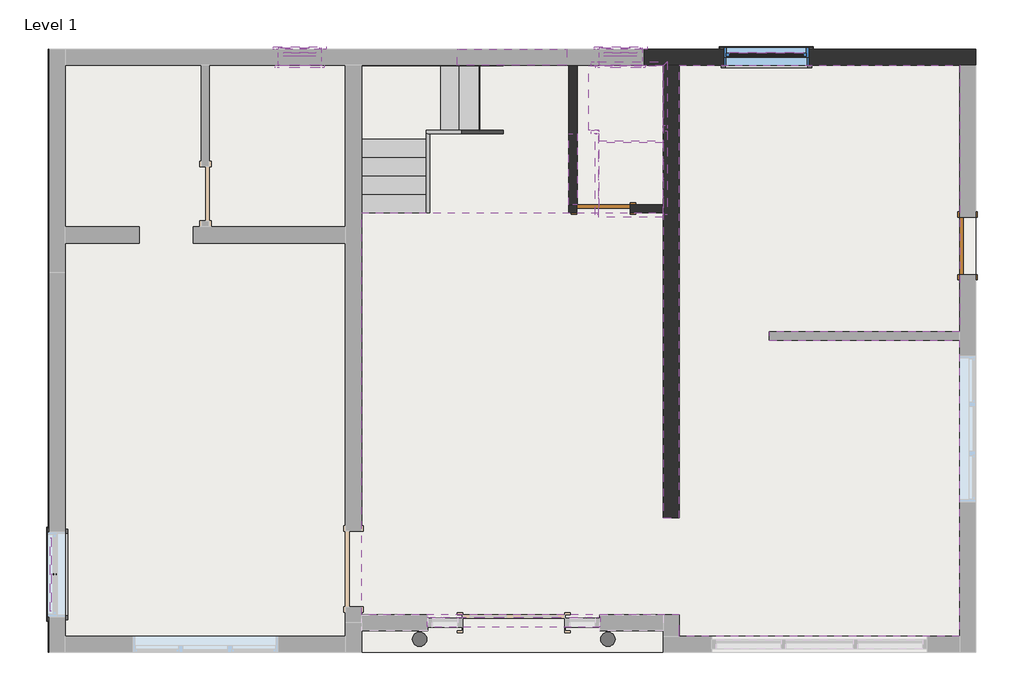
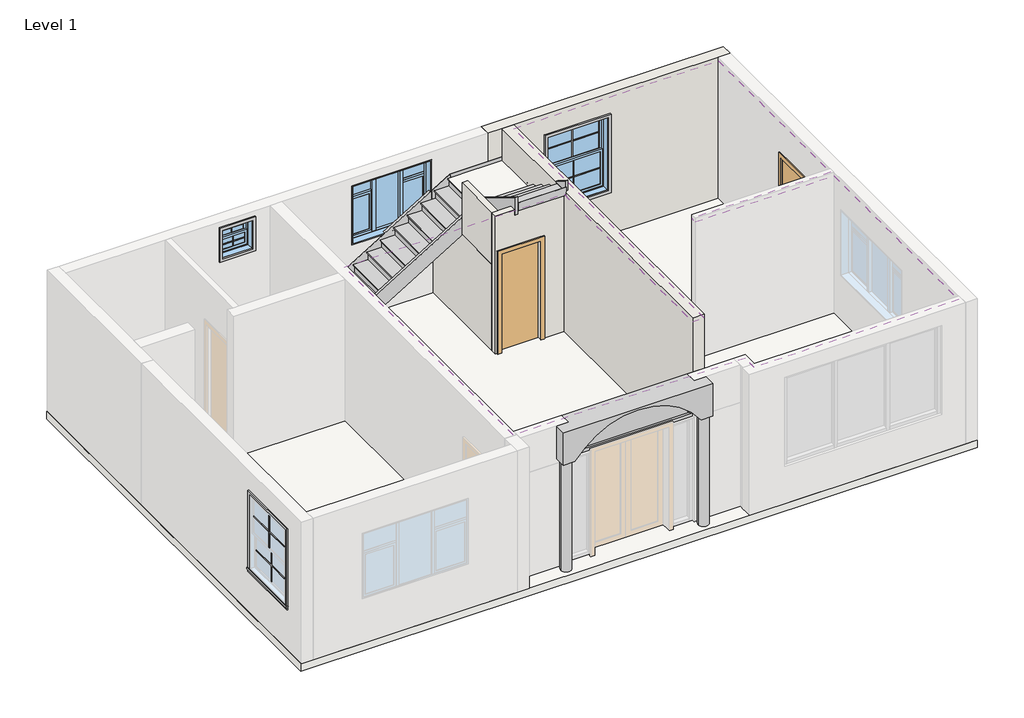
# One storey, part 2 of 2: 18 proxies, 11 members, 5 walls, 4 windows, 3 slabs, 3 stair flights, 2 doors, 1 covering.
"""IFC4 building model written with IfcOpenShell, lengths in millimetres."""

from ifc_helpers import new_model, si_unit, frame, origin, place, context, project, spatial, polyline, outline, extrude, faceted_brep, transform, mapped, element, save
from components import generic_models_1_generic_models_1_1dae4af3, generic_models_2_generic_models_2_701112c8, muntin_pattern_2x2_muntin_pattern_2x2_872d1288, muntin_pattern_2x2_muntin_pattern_2x2_cfeb24ad, trim_window_exterior_flat_with_sill_c3105ee7, trim_window_exterior_flat_with_sill_858dc10d, trim_window_interior_flat_picture_frame_d5efd988, trim_window_interior_flat_picture_frame_3927330c, door_f2b275c1, door_7b345704, non_monolithic_landing_e8e8d04f, non_monolithic_landing_bb3beaf2, stair_flight_8f72ff29, stair_flight_55fbbb17, stair_flight_157d76c2, window_1a7cbd99, window_double_hung_2_x2_15b2d83c, window_double_hung_3_11_b20011b0

model = new_model("IFC4")

# Units and contexts
model_context = context("Model", 3, world=origin())
ifc_project = project(units=[si_unit("LENGTHUNIT", "METRE", prefix="MILLI")], contexts=[model_context])

# Site, building, storey
site = spatial("IfcSite", under=ifc_project)
building = spatial("IfcBuilding", under=site)
storey = spatial("IfcBuildingStorey", under=building, Name="Level 1", Elevation=0.0)

# Proxies
placement = place(None, origin())
generic_models_1_generic_models_1_shape = generic_models_1_generic_models_1_1dae4af3(model_context)
element("IfcBuildingElementProxy", 1, Name="Generic Models 1 : Generic Models 1", ObjectType="Generic Models 1 : Generic Models 1", at=placement, inside=storey, context=model_context, shape_type="MappedRepresentation", body=[
    mapped(generic_models_1_generic_models_1_shape, transform((0.0, 0.0, 0.0), x_axis=(1.0, 0.0, 0.0), y_axis=(0.0, 1.0, 0.0), z_axis=(0.0, 0.0, 1.0))),
])
generic_models_2_generic_models_2_shape = generic_models_2_generic_models_2_701112c8(model_context)
element("IfcBuildingElementProxy", 2, Name="Generic Models 2 : Generic Models 2", ObjectType="Generic Models 2 : Generic Models 2", at=placement, inside=storey, context=model_context, shape_type="MappedRepresentation", body=[
    mapped(generic_models_2_generic_models_2_shape, transform((0.0, 0.0, 0.0), x_axis=(1.0, 0.0, 0.0), y_axis=(0.0, 1.0, 0.0), z_axis=(0.0, 0.0, 1.0))),
])
muntin_pattern_2x2_muntin_pattern_2x2_shape = muntin_pattern_2x2_muntin_pattern_2x2_872d1288(model_context)
element("IfcBuildingElementProxy", 3, Name="Muntin Pattern_2x2 : Muntin Pattern_2x2", ObjectType="Muntin Pattern_2x2 : Muntin Pattern_2x2", at=placement, inside=storey, context=model_context, shape_type="MappedRepresentation", body=[
    mapped(muntin_pattern_2x2_muntin_pattern_2x2_shape, transform((-19390.8072207, 4603.0962903, 1698.625), x_axis=(0.0, 1.0, 0.0), y_axis=(-1.0, 0.0, 0.0), z_axis=(0.0, 0.0, 1.0))),
])
element("IfcBuildingElementProxy", 4, Name="Muntin Pattern_2x2 : Muntin Pattern_2x2", ObjectType="Muntin Pattern_2x2 : Muntin Pattern_2x2", at=placement, inside=storey, context=model_context, shape_type="MappedRepresentation", body=[
    mapped(muntin_pattern_2x2_muntin_pattern_2x2_shape, transform((-19346.3572207, 4603.0962903, 990.6), x_axis=(0.0, 1.0, 0.0), y_axis=(-1.0, 0.0, 0.0), z_axis=(0.0, 0.0, 1.0))),
])
element("IfcBuildingElementProxy", 5, Name="Muntin Pattern_2x2 : Muntin Pattern_2x2", ObjectType="Muntin Pattern_2x2 : Muntin Pattern_2x2", at=placement, inside=storey, context=model_context, shape_type="MappedRepresentation", body=[
    mapped(muntin_pattern_2x2_muntin_pattern_2x2_shape, transform((-9277.2026022, 11998.6707578, 1698.625), x_axis=(1.0, 0.0, 0.0), y_axis=(0.0, 1.0, 0.0), z_axis=(0.0, 0.0, 1.0))),
])
element("IfcBuildingElementProxy", 6, Name="Muntin Pattern_2x2 : Muntin Pattern_2x2", ObjectType="Muntin Pattern_2x2 : Muntin Pattern_2x2", at=placement, inside=storey, context=model_context, shape_type="MappedRepresentation", body=[
    mapped(muntin_pattern_2x2_muntin_pattern_2x2_shape, transform((-9277.2026022, 11954.2207578, 990.6), x_axis=(1.0, 0.0, 0.0), y_axis=(0.0, 1.0, 0.0), z_axis=(0.0, 0.0, 1.0))),
])
muntin_pattern_2x2_muntin_pattern_2x2_2_shape = muntin_pattern_2x2_muntin_pattern_2x2_cfeb24ad(model_context)
element("IfcBuildingElementProxy", 7, Name="Muntin Pattern_2x2 : Muntin Pattern_2x2", ObjectType="Muntin Pattern_2x2 : Muntin Pattern_2x2", at=placement, inside=storey, context=model_context, shape_type="MappedRepresentation", body=[
    mapped(muntin_pattern_2x2_muntin_pattern_2x2_2_shape, transform((-15881.0556236, 11998.6707578, 2460.625), x_axis=(1.0, 0.0, 0.0), y_axis=(0.0, 1.0, 0.0), z_axis=(0.0, 0.0, 1.0))),
])
element("IfcBuildingElementProxy", 8, Name="Muntin Pattern_2x2 : Muntin Pattern_2x2", ObjectType="Muntin Pattern_2x2 : Muntin Pattern_2x2", at=placement, inside=storey, context=model_context, shape_type="MappedRepresentation", body=[
    mapped(muntin_pattern_2x2_muntin_pattern_2x2_2_shape, transform((-15881.0556236, 11954.2207578, 2209.8), x_axis=(1.0, 0.0, 0.0), y_axis=(0.0, 1.0, 0.0), z_axis=(0.0, 0.0, 1.0))),
])
element("IfcBuildingElementProxy", 9, Name="Muntin Pattern_2x2 : Muntin Pattern_2x2", ObjectType="Muntin Pattern_2x2 : Muntin Pattern_2x2", at=placement, inside=storey, context=model_context, shape_type="MappedRepresentation", body=[
    mapped(muntin_pattern_2x2_muntin_pattern_2x2_2_shape, transform((-11339.7531945, 11998.6707578, 1851.025), x_axis=(1.0, 0.0, 0.0), y_axis=(0.0, 1.0, 0.0), z_axis=(0.0, 0.0, 1.0))),
])
element("IfcBuildingElementProxy", 10, Name="Muntin Pattern_2x2 : Muntin Pattern_2x2", ObjectType="Muntin Pattern_2x2 : Muntin Pattern_2x2", at=placement, inside=storey, context=model_context, shape_type="MappedRepresentation", body=[
    mapped(muntin_pattern_2x2_muntin_pattern_2x2_2_shape, transform((-11339.7531945, 11954.2207578, 1600.2), x_axis=(1.0, 0.0, 0.0), y_axis=(0.0, 1.0, 0.0), z_axis=(0.0, 0.0, 1.0))),
])
trim_window_exterior_flat_with_sill_shape = trim_window_exterior_flat_with_sill_c3105ee7(model_context)
element("IfcBuildingElementProxy", 11, Name="Trim-Window-Exterior-Flat : with Sill", ObjectType="Trim-Window-Exterior-Flat : with Sill", at=placement, inside=storey, context=model_context, shape_type="MappedRepresentation", body=[
    mapped(trim_window_exterior_flat_with_sill_shape, transform((-19425.7322207, 4603.0962903, 2438.4), x_axis=(0.0, -1.0, 0.0), y_axis=(0.0, 0.0, 1.0), z_axis=(-1.0, 0.0, 0.0))),
])
element("IfcBuildingElementProxy", 12, Name="Trim-Window-Exterior-Flat : with Sill", ObjectType="Trim-Window-Exterior-Flat : with Sill", at=placement, inside=storey, context=model_context, shape_type="MappedRepresentation", body=[
    mapped(trim_window_exterior_flat_with_sill_shape, transform((-9277.2026022, 12033.5957578, 2438.4), x_axis=(-1.0, 0.0, 0.0), y_axis=(0.0, 0.0, 1.0), z_axis=(0.0, 1.0, 0.0))),
])
trim_window_exterior_flat_with_sill_2_shape = trim_window_exterior_flat_with_sill_858dc10d(model_context)
element("IfcBuildingElementProxy", 13, Name="Trim-Window-Exterior-Flat : with Sill", ObjectType="Trim-Window-Exterior-Flat : with Sill", at=placement, inside=storey, context=model_context, shape_type="MappedRepresentation", body=[
    mapped(trim_window_exterior_flat_with_sill_2_shape, transform((-15881.0556236, 12033.5957578, 2743.2), x_axis=(-1.0, 0.0, 0.0), y_axis=(0.0, 0.0, 1.0), z_axis=(0.0, 1.0, 0.0))),
])
element("IfcBuildingElementProxy", 14, Name="Trim-Window-Exterior-Flat : with Sill", ObjectType="Trim-Window-Exterior-Flat : with Sill", at=placement, inside=storey, context=model_context, shape_type="MappedRepresentation", body=[
    mapped(trim_window_exterior_flat_with_sill_2_shape, transform((-11339.7531945, 12033.5957578, 2133.6), x_axis=(-1.0, 0.0, 0.0), y_axis=(0.0, 0.0, 1.0), z_axis=(0.0, 1.0, 0.0))),
])
trim_window_interior_flat_picture_frame_shape = trim_window_interior_flat_picture_frame_d5efd988(model_context)
element("IfcBuildingElementProxy", 15, Name="Trim-Window-Interior-Flat : Picture Frame", ObjectType="Trim-Window-Interior-Flat : Picture Frame", at=placement, inside=storey, context=model_context, shape_type="MappedRepresentation", body=[
    mapped(trim_window_interior_flat_picture_frame_shape, transform((-19197.1322207, 4603.0962903, 2438.4), x_axis=(0.0, 1.0, 0.0), y_axis=(0.0, 0.0, 1.0), z_axis=(1.0, 0.0, 0.0))),
])
element("IfcBuildingElementProxy", 16, Name="Trim-Window-Interior-Flat : Picture Frame", ObjectType="Trim-Window-Interior-Flat : Picture Frame", at=placement, inside=storey, context=model_context, shape_type="MappedRepresentation", body=[
    mapped(trim_window_interior_flat_picture_frame_shape, transform((-9277.2026022, 11804.9957578, 2438.4), x_axis=(1.0, 0.0, 0.0), y_axis=(0.0, 0.0, 1.0), z_axis=(0.0, -1.0, 0.0))),
])
trim_window_interior_flat_picture_frame_2_shape = trim_window_interior_flat_picture_frame_3927330c(model_context)
element("IfcBuildingElementProxy", 17, Name="Trim-Window-Interior-Flat : Picture Frame", ObjectType="Trim-Window-Interior-Flat : Picture Frame", at=placement, inside=storey, context=model_context, shape_type="MappedRepresentation", body=[
    mapped(trim_window_interior_flat_picture_frame_2_shape, transform((-15881.0556236, 11804.9957578, 2743.2), x_axis=(1.0, 0.0, 0.0), y_axis=(0.0, 0.0, 1.0), z_axis=(0.0, -1.0, 0.0))),
])
element("IfcBuildingElementProxy", 18, Name="Trim-Window-Interior-Flat : Picture Frame", ObjectType="Trim-Window-Interior-Flat : Picture Frame", at=placement, inside=storey, context=model_context, shape_type="MappedRepresentation", body=[
    mapped(trim_window_interior_flat_picture_frame_2_shape, transform((-11339.7531945, 11804.9957578, 2133.6), x_axis=(1.0, 0.0, 0.0), y_axis=(0.0, 0.0, 1.0), z_axis=(0.0, -1.0, 0.0))),
])

# Covering
element("IfcCovering", 19, ObjectType="2' x 4' ACT System", at=placement, inside=storey, context=model_context, shape_type="SweptSolid", body=[
    extrude(outline(polyline([(-19197.1322207, 9290.2207935), (-18149.1852461, 9290.2207935), (-18149.1852461, 9518.8207935), (-19197.1322207, 9518.8207935), (-19197.1322207, 11804.9957578), (-17272.3740665, 11804.9957578), (-17272.3740665, 9518.8207935), (-17388.0183685, 9518.8207935), (-17388.0183685, 9290.2207935), (-15233.3556236, 9290.2207935), (-15233.3556236, 3726.7962903), (-19197.1322207, 3726.7962903), (-19197.1322207, 9290.2207935)])), frame((0.0, 0.0, 2819.4), z_axis=(0.0, 0.0, 1.0), x_axis=(1.0, 0.0, 0.0)), (0.0, 0.0, 1.0), 57.15),
    extrude(outline(polyline([(-6543.9817031, 11804.9957578), (-6543.9817031, 8032.8333114), (-9237.1629596, 8032.8333114), (-9237.1629596, 7918.5333114), (-6545.326005, 7918.5333114), (-6545.326005, 3726.7962903), (-10507.7583002, 3726.7962903), (-10507.7583002, 4031.4170165), (-15004.7556236, 4031.4170165), (-15004.7556236, 9720.1872586), (-10737.7026022, 9720.1872586), (-10737.7026022, 5401.1206207), (-10509.1026022, 5401.1206207), (-10509.1026022, 11804.9957578), (-6543.9817031, 11804.9957578)])), frame((0.0, 0.0, 2819.4), z_axis=(0.0, 0.0, 1.0), x_axis=(1.0, 0.0, 0.0)), (0.0, 0.0, 1.0), 57.15),
])

# Doors
door_shape = door_f2b275c1(model_context)
element("IfcDoor", 20, ObjectType="Single-Flush : 30\" x 80\"", at=placement, inside=storey, context=model_context, shape_type="MappedRepresentation", body=[
    mapped(door_shape, transform((-11582.1099332, 9778.180515, 0.0), x_axis=(-1.0, 0.0, 0.0), y_axis=(0.0, -1.0, 0.0), z_axis=(0.0, 0.0, 1.0))),
])
door_2_shape = door_7b345704(model_context)
element("IfcDoor", 21, ObjectType="Single-Flush : 32\" x 84\"", at=placement, inside=storey, context=model_context, shape_type="MappedRepresentation", body=[
    mapped(door_2_shape, transform((-6429.6817031, 9252.2957578, 0.0), x_axis=(0.0, -1.0, 0.0), y_axis=(1.0, 0.0, 0.0), z_axis=(0.0, 0.0, 1.0))),
])

# Members
element("IfcMember", 22, ObjectType="Stringer - 2\" Width", at=placement, inside=storey, context=model_context, shape_type="SweptSolid", body=[
    extrude(outline(polyline([(9720.1872586, 0.0), (9720.1872586, 212.7786153), (10805.6326245, 878.3052632), (10891.6353161, 573.5052632), (9956.2728747, 0.0), (9720.1872586, 0.0)])), frame((-15055.3982861, 0.0, 0.0), z_axis=(1.0, 0.0, 0.0), x_axis=(0.0, 1.0, 0.0)), (0.0, 0.0, 1.0), 50.8),
])
element("IfcMember", 23, ObjectType="Stringer - 2\" Width", at=placement, inside=storey, context=model_context, shape_type="SweptSolid", body=[
    extrude(outline(polyline([(9720.1872586, 0.0), (9720.1872586, 212.7786153), (10838.2453953, 898.3013576), (10838.2453953, 540.7699306), (9956.2728747, 0.0), (9720.1872586, 0.0)])), frame((-14090.1982861, 0.0, 0.0), z_axis=(1.0, 0.0, 0.0), x_axis=(0.0, 1.0, 0.0)), (0.0, 0.0, 1.0), 50.8),
])
element("IfcMember", 24, ObjectType="Stringer - 2\" Width", at=placement, inside=storey, context=model_context, shape_type="SweptSolid", body=[
    extrude(outline(polyline([(878.3052632, -14109.3311056), (573.5052632, -14023.328414), (2017.2947368, -11668.5698202), (2322.0947368, -11754.5725119), (878.3052632, -14109.3311056)])), frame((0.0, 11803.4453953, 0.0), z_axis=(0.0, 1.0, 0.0), x_axis=(0.0, 0.0, 1.0)), (0.0, 0.0, 1.0), 50.8),
])
element("IfcMember", 25, ObjectType="Stringer - 2\" Width", at=placement, inside=storey, context=model_context, shape_type="SweptSolid", body=[
    extrude(outline(polyline([(890.0363015, -14090.1982861), (532.5048745, -14090.1982861), (2017.2947368, -11668.5698202), (2322.0947368, -11754.5725119), (890.0363015, -14090.1982861)])), frame((0.0, 10838.2453953, 0.0), z_axis=(0.0, 1.0, 0.0), x_axis=(0.0, 0.0, 1.0)), (0.0, 0.0, 1.0), 50.8),
])
element("IfcMember", 26, ObjectType="Stringer - 2\" Width", at=placement, inside=storey, context=model_context, shape_type="Brep", body=[
    faceted_brep([(-14109.3311056, 11803.4453953, 878.3052632), (-14109.3311056, 11854.2453953, 878.3052632), (-15055.3982861, 11854.2453953, 878.3052632), (-15004.5982861, 11803.4453953, 878.3052632), (-14023.328414, 11803.4453953, 573.5052632), (-15004.5982861, 11803.4453953, 573.5052632), (-14023.328414, 11854.2453953, 573.5052632), (-15055.3982861, 11854.2453953, 573.5052632)], [[[0, 1, 2, 3]], [[4, 0, 3, 5]], [[6, 4, 5, 7]], [[1, 6, 7, 2]], [[1, 0, 4, 6]], [[2, 7, 5, 3]]]),
])
element("IfcMember", 27, ObjectType="Stringer - 2\" Width", at=placement, inside=storey, context=model_context, shape_type="Brep", body=[
    faceted_brep([(-15004.5982861, 11803.4453953, 878.3052632), (-15055.3982861, 11854.2453953, 878.3052632), (-15055.3982861, 10805.6326245, 878.3052632), (-15004.5982861, 10805.6326245, 878.3052632), (-15004.5982861, 11803.4453953, 573.5052632), (-15004.5982861, 10891.6353161, 573.5052632), (-15055.3982861, 11854.2453953, 573.5052632), (-15055.3982861, 10891.6353161, 573.5052632)], [[[0, 1, 2, 3]], [[4, 0, 3, 5]], [[6, 4, 5, 7]], [[1, 6, 7, 2]], [[1, 0, 4, 6]], [[2, 7, 5, 3]]]),
])
element("IfcMember", 28, ObjectType="Stringer - 2\" Width", at=placement, inside=storey, context=model_context, shape_type="SweptSolid", body=[
    extrude(outline(polyline([(10959.0950804, 2322.0947368), (10873.0923887, 2017.2947368), (9689.7818525, 2742.8261356), (9689.7818525, 3100.3575626), (10959.0950804, 2322.0947368)])), frame((-10733.9149392, 0.0, 0.0), z_axis=(1.0, 0.0, 0.0), x_axis=(0.0, 1.0, 0.0)), (0.0, 0.0, 1.0), 50.8),
])
element("IfcMember", 29, ObjectType="Stringer - 2\" Width", at=placement, inside=storey, context=model_context, shape_type="SweptSolid", body=[
    extrude(outline(polyline([(10838.2453953, 2396.1921427), (10838.2453953, 2038.6607157), (9689.7818525, 2742.8261356), (9689.7818525, 3100.3575626), (10838.2453953, 2396.1921427)])), frame((-11699.1149392, 0.0, 0.0), z_axis=(1.0, 0.0, 0.0), x_axis=(0.0, 1.0, 0.0)), (0.0, 0.0, 1.0), 50.8),
])
element("IfcMember", 30, ObjectType="Stringer - 2\" Width", at=placement, inside=storey, context=model_context, shape_type="Brep", body=[
    faceted_brep([(-10733.9149392, 10959.0950804, 2322.0947368), (-10683.1149392, 10959.0950804, 2322.0947368), (-10683.1149392, 11854.2453953, 2322.0947368), (-10733.9149392, 11803.4453953, 2322.0947368), (-10733.9149392, 10873.0923887, 2017.2947368), (-10733.9149392, 11803.4453953, 2017.2947368), (-10683.1149392, 10873.0923887, 2017.2947368), (-10683.1149392, 11854.2453953, 2017.2947368)], [[[0, 1, 2, 3]], [[4, 0, 3, 5]], [[6, 4, 5, 7]], [[1, 6, 7, 2]], [[1, 0, 4, 6]], [[2, 7, 5, 3]]]),
])
element("IfcMember", 31, ObjectType="Stringer - 2\" Width", at=placement, inside=storey, context=model_context, shape_type="Brep", body=[
    faceted_brep([(-10733.9149392, 11803.4453953, 2322.0947368), (-10683.1149392, 11854.2453953, 2322.0947368), (-11754.5725119, 11854.2453953, 2322.0947368), (-11754.5725119, 11803.4453953, 2322.0947368), (-10733.9149392, 11803.4453953, 2017.2947368), (-11668.5698202, 11803.4453953, 2017.2947368), (-10683.1149392, 11854.2453953, 2017.2947368), (-11668.5698202, 11854.2453953, 2017.2947368)], [[[0, 1, 2, 3]], [[4, 0, 3, 5]], [[6, 4, 5, 7]], [[1, 6, 7, 2]], [[1, 0, 4, 6]], [[2, 7, 5, 3]]]),
])
element("IfcMember", 32, ObjectType="Stringer - 2\" Width", at=placement, inside=storey, context=model_context, shape_type="SweptSolid", body=[
    extrude(outline(polyline([(2322.0947368, -11754.5725119), (2017.2947368, -11668.5698202), (2017.2947368, -11648.3149392), (2322.0947368, -11648.3149392), (2322.0947368, -11754.5725119)])), frame((0.0, 10838.2453953, 0.0), z_axis=(0.0, 1.0, 0.0), x_axis=(0.0, 0.0, 1.0)), (0.0, 0.0, 1.0), 50.8),
])

# Slabs
element("IfcSlab", 33, ObjectType="6\"", at=placement, inside=storey, context=model_context, shape_type="SweptSolid", body=[
    extrude(outline(polyline([(-6312.7810046, 12034.9129661), (-6312.7810046, 3498.1962903), (-19437.2989325, 3498.1962903), (-19437.2989325, 12034.9129661), (-6312.7810046, 12034.9129661)])), frame((0.0, 0.0, -152.4), z_axis=(0.0, 0.0, 1.0), x_axis=(1.0, 0.0, 0.0)), (0.0, 0.0, 1.0), 152.4),
])
non_monolithic_landing_shape = non_monolithic_landing_e8e8d04f(model_context)
element("IfcSlab", 34, ObjectType="Non-Monolithic Landing", at=placement, inside=storey, context=model_context, shape_type="MappedRepresentation", body=[
    mapped(non_monolithic_landing_shape, transform((0.0, 0.0, 0.0), x_axis=(1.0, 0.0, 0.0), y_axis=(0.0, 1.0, 0.0), z_axis=(0.0, 0.0, 1.0))),
])
non_monolithic_landing_2_shape = non_monolithic_landing_bb3beaf2(model_context)
element("IfcSlab", 35, ObjectType="Non-Monolithic Landing", at=placement, inside=storey, context=model_context, shape_type="MappedRepresentation", body=[
    mapped(non_monolithic_landing_2_shape, transform((0.0, 0.0, 0.0), x_axis=(1.0, 0.0, 0.0), y_axis=(0.0, 1.0, 0.0), z_axis=(0.0, 0.0, 1.0))),
])

# Stair flights
stair_flight_shape = stair_flight_8f72ff29(model_context)
element("IfcStairFlight", 36, ObjectType="2\" Tread 1\" Nosing 1/4\" Riser", at=placement, inside=storey, context=model_context, shape_type="MappedRepresentation", body=[
    mapped(stair_flight_shape, transform((0.0, 0.0, 0.0), x_axis=(1.0, 0.0, 0.0), y_axis=(0.0, 1.0, 0.0), z_axis=(0.0, 0.0, 1.0))),
])
stair_flight_2_shape = stair_flight_55fbbb17(model_context)
element("IfcStairFlight", 37, ObjectType="2\" Tread 1\" Nosing 1/4\" Riser", at=placement, inside=storey, context=model_context, shape_type="MappedRepresentation", body=[
    mapped(stair_flight_2_shape, transform((0.0, 0.0, 0.0), x_axis=(1.0, 0.0, 0.0), y_axis=(0.0, 1.0, 0.0), z_axis=(0.0, 0.0, 1.0))),
])
stair_flight_3_shape = stair_flight_157d76c2(model_context)
element("IfcStairFlight", 38, ObjectType="2\" Tread 1\" Nosing 1/4\" Riser", at=placement, inside=storey, context=model_context, shape_type="MappedRepresentation", body=[
    mapped(stair_flight_3_shape, transform((0.0, 0.0, 0.0), x_axis=(1.0, 0.0, 0.0), y_axis=(0.0, 1.0, 0.0), z_axis=(0.0, 0.0, 1.0))),
])

# Walls
element("IfcWall", 39, ObjectType="4.5\"", at=placement, inside=storey, context=model_context, shape_type="Brep", body=[
    faceted_brep([(-11963.1099332, 9835.330515, 2032.0), (-11963.1099332, 9835.330515, 0.0), (-12071.0599332, 9835.330515, 0.0), (-12071.0599332, 9835.330515, 1772.0676647), (-12071.0599332, 9835.330515, 2836.7789474), (-10737.7026022, 9835.330515, 2836.7789474), (-10737.7026022, 9835.330515, 0.0), (-11201.1099332, 9835.330515, 0.0), (-11201.1099332, 9835.330515, 2032.0), (-12071.0599332, 9721.030515, 0.0), (-11963.1099332, 9721.030515, 0.0), (-11963.1099332, 9721.030515, 2032.0), (-11201.1099332, 9721.030515, 2032.0), (-11201.1099332, 9721.030515, 0.0), (-10737.7026022, 9721.030515, 0.0), (-10737.7026022, 9721.030515, 2836.7789474), (-12071.0599332, 9721.030515, 2836.7789474)], [[[0, 1, 2, 3, 4, 5, 6, 7, 8]], [[9, 10, 11, 12, 13, 14, 15, 16]], [[7, 6, 14, 13]], [[2, 1, 10, 9]], [[5, 4, 16, 15]], [[6, 5, 15, 14]], [[2, 9, 16, 4, 3]], [[11, 10, 1, 0]], [[12, 11, 0, 8]], [[13, 12, 8, 7]]]),
])
element("IfcWall", 40, ObjectType="4.5\"", at=placement, inside=storey, context=model_context, shape_type="Brep", body=[
    faceted_brep([(-11956.7599332, 9835.330515, 0.0), (-11956.7599332, 11804.9957578, 0.0), (-11956.7599332, 11804.9957578, 1772.0676647), (-11956.7599332, 10838.2453953, 1772.0676647), (-11956.7599332, 9835.330515, 1772.0676647), (-12071.0599332, 9835.330515, 0.0), (-12071.0599332, 9835.330515, 1772.0676647), (-12071.0599332, 10838.2453953, 1772.0676647), (-12071.0599332, 11804.9957578, 1772.0676647), (-12071.0599332, 11804.9957578, 0.0)], [[[0, 1, 2, 3, 4]], [[5, 6, 7, 8, 9]], [[1, 0, 5, 9]], [[4, 3, 2, 8, 7, 6]], [[2, 1, 9, 8]], [[0, 4, 6, 5]]]),
])
element("IfcWall", 41, ObjectType="4.5\"", at=placement, inside=storey, context=model_context, shape_type="Brep", body=[
    faceted_brep([(-12071.0599332, 10838.2453953, 1772.0676647), (-12071.0599332, 9835.330515, 1772.0676647), (-12071.0599332, 9835.330515, 2836.7789474), (-12071.0599332, 9835.330515, 2839.9177191), (-12071.0599332, 10838.2453953, 2839.9177191), (-11956.7599332, 10838.2453953, 1772.0676647), (-11956.7599332, 10838.2453953, 2839.9177191), (-11956.7599332, 9835.330515, 2839.9177191), (-11956.7599332, 9835.330515, 1772.0676647)], [[[0, 1, 2, 3, 4]], [[5, 6, 7, 8]], [[1, 0, 5, 8]], [[4, 3, 7, 6]], [[0, 4, 6, 5]], [[3, 2, 1, 8, 7]]]),
])
element("IfcWall", 42, ObjectType="9\"", at=placement, inside=storey, context=model_context, shape_type="Brep", body=[
    faceted_brep([(-6315.3817031, 12033.5957578, 0.0), (-11009.5531945, 12033.5957578, 0.0), (-11009.5531945, 12033.5957578, 2895.6), (-6315.3817031, 12033.5957578, 2895.6), (-9874.1026022, 12033.5957578, 2438.4), (-9874.1026022, 12033.5957578, 914.4), (-8680.3026022, 12033.5957578, 914.4), (-8680.3026022, 12033.5957578, 2438.4), (-6315.3817031, 11804.9957578, 0.0), (-6315.3817031, 11804.9957578, 2895.6), (-6543.9817031, 11804.9957578, 2895.6), (-10509.1026022, 11804.9957578, 2895.6), (-10737.7026022, 11804.9957578, 2895.6), (-11009.5531945, 11804.9957578, 2895.6), (-11009.5531945, 11804.9957578, 0.0), (-10737.7026022, 11804.9957578, 0.0), (-10509.1026022, 11804.9957578, 0.0), (-6543.9817031, 11804.9957578, 0.0), (-9874.1026022, 11804.9957578, 2438.4), (-8680.3026022, 11804.9957578, 2438.4), (-8680.3026022, 11804.9957578, 914.4), (-9874.1026022, 11804.9957578, 914.4)], [[[0, 1, 2, 3], [4, 5, 6, 7]], [[8, 9, 10, 11, 12, 13, 14, 15, 16, 17], [18, 19, 20, 21]], [[1, 0, 8, 17, 16, 15, 14]], [[2, 1, 14, 13]], [[3, 2, 13, 12, 11, 10, 9]], [[0, 3, 9, 8]], [[5, 4, 18, 21]], [[6, 5, 21, 20]], [[7, 6, 20, 19]], [[4, 7, 19, 18]]]),
])
element("IfcWall", 43, ObjectType="9\"", at=placement, inside=storey, context=model_context, shape_type="Brep", body=[
    faceted_brep([(-10737.7026022, 11804.9957578, 0.0), (-10737.7026022, 9835.330515, 0.0), (-10737.7026022, 9721.030515, 0.0), (-10737.7026022, 5401.1206207, 0.0), (-10737.7026022, 5401.1206207, 2895.6), (-10737.7026022, 11804.9957578, 2895.6), (-10509.1026022, 11804.9957578, 0.0), (-10509.1026022, 11804.9957578, 2895.6), (-10509.1026022, 5401.1206207, 2895.6), (-10509.1026022, 5401.1206207, 0.0)], [[[0, 1, 2, 3, 4, 5]], [[6, 7, 8, 9]], [[3, 2, 1, 0, 6, 9]], [[4, 3, 9, 8]], [[5, 4, 8, 7]], [[0, 5, 7, 6]]]),
])

# Windows
window_shape = window_1a7cbd99(model_context)
element("IfcWindow", 44, ObjectType="Window-Casement-Triple-Side-Transom : 61\" x 48\"", at=placement, inside=storey, context=model_context, shape_type="MappedRepresentation", body=[
    mapped(window_shape, transform((-12877.5099332, 11919.2957578, 609.6), x_axis=(1.0, 0.0, 0.0), y_axis=(0.0, 1.0, 0.0), z_axis=(0.0, 0.0, 1.0))),
])
window_double_hung_2_x2_shape = window_double_hung_2_x2_15b2d83c(model_context)
element("IfcWindow", 45, ObjectType="Window-Double-Hung : 2'x2'", at=placement, inside=storey, context=model_context, shape_type="MappedRepresentation", body=[
    mapped(window_double_hung_2_x2_shape, transform((-15881.0556236, 11919.2957578, 1219.2), x_axis=(1.0, 0.0, 0.0), y_axis=(0.0, 1.0, 0.0), z_axis=(0.0, 0.0, 1.0))),
])
element("IfcWindow", 46, ObjectType="Window-Double-Hung : 2'x2'", at=placement, inside=storey, context=model_context, shape_type="MappedRepresentation", body=[
    mapped(window_double_hung_2_x2_shape, transform((-11339.7531945, 11919.2957578, 609.6), x_axis=(1.0, 0.0, 0.0), y_axis=(0.0, 1.0, 0.0), z_axis=(0.0, 0.0, 1.0))),
])
window_double_hung_3_11_shape = window_double_hung_3_11_b20011b0(model_context)
element("IfcWindow", 47, ObjectType="Window-Double-Hung : 3'11", at=placement, inside=storey, context=model_context, shape_type="MappedRepresentation", body=[
    mapped(window_double_hung_3_11_shape, transform((-9277.2026022, 11919.2957578, 0.0), x_axis=(1.0, 0.0, 0.0), y_axis=(0.0, 1.0, 0.0), z_axis=(0.0, 0.0, 1.0))),
])

save(model, "model.ifc")

# Revit data of these elements
# Type "Muntin Pattern_2x2 : Muntin Pattern_2x2"
#   Width [instance default] = 4' - 0"
#   Thickness = 0' - 0 1/2"
#   Height [instance default] = 4' - 0"
#   Distance = 0' - 0 3/4"
#   Interior Material [instance default] = none
#   Exterior Material [instance default] = none
#   Default Elevation = 0
# Type "Trim-Window-Exterior-Flat : with Sill"
#   Trim Width = 0' - 2 1/4"
#   Trim Thickness_Picture Frame = 0' - 1 1/4"
#   Trim Thickness_with Sill = 0' - 0 3/4"
#   Sill Thickness = 0' - 1 1/4"
#   Opening Width [instance default] = 2' - 0"
#   Opening Height [instance default] = 3' - 0"
#   Default Elevation = 4' - 0"
#   Sill = yes
#   Picture Frame = no
#   Trim Material [instance default] = none
# Type "Trim-Window-Interior-Flat : Picture Frame"
#   Trim Thickness_Picture Frame = 0' - 1 1/4"
#   Trim Width = 0' - 2 1/4"
#   Trim Thickness_with Sill = 0' - 0 3/4"
#   Sill Thickness = 0' - 1 1/4"
#   Opening Width [instance default] = 2' - 0"
#   Opening Height [instance default] = 3' - 0"
#   Default Elevation = 4' - 0"
#   Sill = no
#   Picture Frame = yes
#   Trim Material [instance default] = none
# Type "2' x 4' ACT System"
#   Assembly Code = "C3030210"
#   built-in parameter 1002203 = 1 (stored number, unit not read)
#   built-in parameter 1002202 = 1 (stored number, unit not read)
#   Layers, outside or top first: 0' - 1 5/8" "Default" (function 1); 0' - 0 5/8" "Acoustic Ceiling Tile 24 x 48" (function 5)
# Type "Single-Flush : 30\" x 80\""
#   Type Mark = "5"
#   Construction Type Id = "MDOOR"
#   Assembly Code = "C1020"
#   Analytic Construction = "Metal"
#   Thickness = 0' - 2"
#   Heat Transfer Coefficient (U) = 0.651978 BTU/(h·ft²·°F)
#   Height = 6' - 8"
#   Trim Projection Ext = 0' - 1"
#   Trim Projection Int = 0' - 1"
#   Trim Width = 0' - 3"
#   Width = 2' - 6"
#   Define Thermal Properties by = 1
#   Define Thermal Properties by = 1
#   Door Material = Door - Panel
#   Frame Material = Door - Frame
#   Visual Light Transmittance = 0
#   Solar Heat Gain Coefficient = 0
#   Function = (empty or 0)
#   Wall Closure = (empty or 0)
# Type "Single-Flush : 32\" x 84\""
#   Type Mark = "3"
#   Construction Type Id = "MDOOR"
#   Assembly Code = "C1020"
#   Analytic Construction = "Metal"
#   Thickness = 0' - 2"
#   Heat Transfer Coefficient (U) = 0.651978 BTU/(h·ft²·°F)
#   Height = 7' - 0"
#   Trim Projection Ext = 0' - 1"
#   Trim Projection Int = 0' - 1"
#   Trim Width = 0' - 3"
#   Width = 2' - 8"
#   Define Thermal Properties by = 1
#   Define Thermal Properties by = 1
#   Door Material = Door - Panel
#   Frame Material = Door - Frame
#   Visual Light Transmittance = 0
#   Solar Heat Gain Coefficient = 0
#   Function = (empty or 0)
#   Wall Closure = (empty or 0)
# Type "6\""
#   Assembly Code = "B1010"
#   Function = 0
#   Layers, outside or top first: 0' - 6" no material (function 1)
# Type "4.5\""
#   Assembly Code = "B2010"
#   Layers, outside or top first: 0' - 4 1/2" no material (function 1)
# Type "9\""
#   Assembly Code = "B2010"
#   Layers, outside or top first: 0' - 9" no material (function 1)
# Type "Window-Casement-Triple-Side-Transom : 61\" x 48\""
#   Type Mark = "23"
#   Fire Rating = "0.5h"
#   Assembly Code = "B2020100"
#   Analytic Construction = "Double glazing - domestic"
#   Window Width = 1' - 8.33333"
#   Window Inset [instance default] = 0' - 0 5/8"
#   Wall Thickness [instance default] = 0' - 6"
#   Visual Light Transmittance = 0.81
#   Transom Height Ratio = 0.3
#   Thermal Resistance (R) = 1.8146 (h·ft²·°F)/BTU
#   Solar Heat Gain Coefficient = 0.76
#   Rough Width = 5' - 1 1/2"
#   Rough Height = 4' - 0 1/2"
#   Open Window Height = 2' - 9.6"
#   Heat Transfer Coefficient (U) = 0.5511 BTU/(h·ft²·°F)
#   Height = 4' - 0"
#   Transom Height = 1' - 2.4"
#   Frame Gap 3 [instance default] = 0' - 1 83/128"
#   Frame Gap 2 [instance default] = 0' - 0 5/8"
#   Frame Gap 1 = 0' - 1 51/128"
#   Default Sill Height = 3' - 0"
#   Width = 5' - 1"
#   Frame Material = Metal - Aluminum
#   Glass Panel Material = Glass
#   Wall Closure = (empty or 0)
# Type "Window-Double-Hung : 2'x2'"
#   Type Mark = "26"
#   Fire Rating = "0.5h"
#   Construction Type Id = "DG-DR"
#   Assembly Code = "B2020100"
#   Analytic Construction = "Double glazing - domestic"
#   Wall Thickness [instance default] = 0' - 6"
#   Window Inset [instance default] = 0' - 0"
#   Visual Light Transmittance = 0.81
#   Thermal Resistance (R) = 1.8146 (h·ft²·°F)/BTU
#   Solar Heat Gain Coefficient = 0.76
#   Muntin Width = 1' - 6"
#   Muntin Height = 0' - 8 1/8"
#   Interior Wall Closure [instance default] = 0' - 1 1/2"
#   Rough Width = 2' - 0 1/2"
#   Rough Height = 2' - 0 1/2"
#   Frame Extension [instance default] = 0' - 1 1/4"
#   Exterior Wall Closure [instance default] = 0' - 0 1/2"
#   Extension Jamb [instance default] = 0' - 1 1/2"
#   Heat Transfer Coefficient (U) = 0.5511 BTU/(h·ft²·°F)
#   Height = 2' - 0"
#   Width = 2' - 0"
#   Top Muntin Visibility = yes
#   Indicator Visibility [instance default] = yes
#   Extension Jamb Visibility [instance default] = yes
#   Interior Trim Visibility [instance default] = yes
#   Exterior Trim Visibility [instance default] = yes
#   Define Thermal Properties by = 1
#   Bottom Muntin Visibility = yes
#   Muntin Pattern = Muntin Pattern_2x2 : Muntin Pattern_2x2
#   Interior Trim Material = Wood - Stained
#   Interior Trim = Trim-Window-Interior-Flat : Picture Frame
#   Exterior Trim Material = Clad - White
#   Exterior Trim = Trim-Window-Exterior-Flat : with Sill
#   Glass Panel Material = Glass
#   Exterior Frame Material = Clad - White
#   Interior Frame Material = Wood - Stained
#   Wall Closure = (empty or 0)
# Type "Window-Double-Hung : 3'11"
#   Type Mark = "21"
#   Fire Rating = "0.5h"
#   Construction Type Id = "DG-DR"
#   Assembly Code = "B2020100"
#   Analytic Construction = "Double glazing - domestic"
#   Wall Thickness [instance default] = 0' - 6"
#   Window Inset [instance default] = 0' - 0"
#   Visual Light Transmittance = 0.81
#   Thermal Resistance (R) = 1.8146 (h·ft²·°F)/BTU
#   Solar Heat Gain Coefficient = 0.76
#   Muntin Width = 3' - 5"
#   Muntin Height = 2' - 2 1/8"
#   Interior Wall Closure [instance default] = 0' - 1 1/2"
#   Rough Width = 3' - 11 1/2"
#   Rough Height = 5' - 0 1/2"
#   Frame Extension [instance default] = 0' - 1 1/4"
#   Exterior Wall Closure [instance default] = 0' - 0 1/2"
#   Extension Jamb [instance default] = 0' - 1 1/2"
#   Heat Transfer Coefficient (U) = 0.5511 BTU/(h·ft²·°F)
#   Height = 5' - 0"
#   Width = 3' - 11"
#   Top Muntin Visibility = yes
#   Indicator Visibility [instance default] = yes
#   Extension Jamb Visibility [instance default] = yes
#   Interior Trim Visibility [instance default] = yes
#   Exterior Trim Visibility [instance default] = yes
#   Define Thermal Properties by = 1
#   Bottom Muntin Visibility = yes
#   Muntin Pattern = Muntin Pattern_2x2 : Muntin Pattern_2x2
#   Interior Trim Material = Wood - Stained
#   Interior Trim = Trim-Window-Interior-Flat : Picture Frame
#   Exterior Trim Material = Clad - White
#   Exterior Trim = Trim-Window-Exterior-Flat : with Sill
#   Glass Panel Material = Glass
#   Exterior Frame Material = Clad - White
#   Interior Frame Material = Wood - Stained
#   Wall Closure = (empty or 0)
# Element 1 (IfcBuildingElementProxy, "Generic Models 1 : Generic Models 1")
#   Phase Created = New Construction
#   Materials on its faces: "Gypsum Wall Board", "Glass"
# Element 2 (IfcBuildingElementProxy, "Generic Models 2 : Generic Models 2")
#   Phase Created = New Construction
# Elements 3, 4, 5, 6 (IfcBuildingElementProxy, "Muntin Pattern_2x2 : Muntin Pattern_2x2")
#   Width = 3' - 5"
#   Height = 2' - 2 1/8"
#   Interior Material = Wood - Stained
#   Exterior Material = Clad - White
#   Phase Created = New Construction
#   Materials on its faces: "Clad - White", "Wood - Stained"
# Elements 7, 8, 9, 10 (IfcBuildingElementProxy, "Muntin Pattern_2x2 : Muntin Pattern_2x2")
#   Width = 1' - 6"
#   Height = 0' - 8 1/8"
#   Interior Material = Wood - Stained
#   Exterior Material = Clad - White
#   Phase Created = New Construction
#   Materials on its faces: "Clad - White", "Wood - Stained"
# Elements 11, 12 (IfcBuildingElementProxy, "Trim-Window-Exterior-Flat : with Sill")
#   Opening Width = 3' - 11"
#   Opening Height = 5' - 0"
#   Trim Material = Clad - White
#   Phase Created = New Construction
#   Materials on its faces: "Clad - White"
# Elements 13, 14 (IfcBuildingElementProxy, "Trim-Window-Exterior-Flat : with Sill")
#   Opening Width = 2' - 0"
#   Opening Height = 2' - 0"
#   Trim Material = Clad - White
#   Phase Created = New Construction
#   Materials on its faces: "Clad - White"
# Elements 15, 16 (IfcBuildingElementProxy, "Trim-Window-Interior-Flat : Picture Frame")
#   Opening Width = 3' - 11"
#   Opening Height = 5' - 0"
#   Trim Material = Wood - Stained
#   Phase Created = New Construction
#   Materials on its faces: "Wood - Stained"
# Elements 17, 18 (IfcBuildingElementProxy, "Trim-Window-Interior-Flat : Picture Frame")
#   Opening Width = 2' - 0"
#   Opening Height = 2' - 0"
#   Trim Material = Wood - Stained
#   Phase Created = New Construction
#   Materials on its faces: "Wood - Stained"
# Element 19 (IfcCovering, "2' x 4' ACT System")
#   Height Offset From Level = 9' - 3"
#   Phase Created = New Construction
#   Materials on its faces: "Acoustic Ceiling Tile 24 x 48", "Default"
# Element 20 (IfcDoor, "Single-Flush : 30\" x 80\"")
#   Phase Created = New Construction
#   Materials on its faces: "Door - Frame", "Door - Panel"
# Element 21 (IfcDoor, "Single-Flush : 32\" x 84\"")
#   Phase Created = New Construction
#   Materials on its faces: "Door - Frame", "Door - Panel"
# Elements 22, 23, 24, 25, 26, 27, 28, 29, 30, 31, 32 (IfcMember, "Stringer - 2\" Width")
#   Phase Created = New Construction
# Element 33 (IfcSlab, "6\"")
#   Height Offset From Level = 0' - 0"
#   Phase Created = New Construction
#   Materials on its faces: "Default Floor"
# Elements 34, 35 (IfcSlab, "Non-Monolithic Landing")
#   Phase Created = New Construction
# Elements 36, 37, 38 (IfcStairFlight, "2\" Tread 1\" Nosing 1/4\" Riser")
#   Phase Created = New Construction
# Element 39 (IfcWall, "4.5\"")
#   Top Offset = -0' - 2.31579"
#   Base Offset = 0' - 0"
#   wall height = 9' - 3.68421"
#   Phase Created = New Construction
#   Base Constraint = Level 1
#   Top Constraint = 1 slab level
#   Materials on its faces: "Default Wall"
# Element 40 (IfcWall, "4.5\"")
#   Top Offset = -3' - 8.23356"
#   Base Offset = 0' - 0"
#   wall height = 5' - 9.76644"
#   Phase Created = New Construction
#   Base Constraint = Level 1
#   Top Constraint = 1 slab level
#   Materials on its faces: "Default Wall"
# Element 41 (IfcWall, "4.5\"")
#   built-in parameter 1001111 = 5' - 9.76644"
#   Top Offset = -0' - 2.19222"
#   Base Offset = 5' - 9.76644"
#   wall height = 3' - 6.04134"
#   Phase Created = New Construction
#   Base Constraint = Level 1
#   Top Constraint = 1 slab level
#   Materials on its faces: "Default Wall"
# Elements 42, 43 (IfcWall, "9\"")
#   Top Offset = 0' - 0"
#   Base Offset = 0' - 0"
#   wall height = 9' - 6"
#   Phase Created = New Construction
#   Base Constraint = Level 1
#   Top Constraint = 1 slab level
#   Materials on its faces: "Default Wall"
# Element 44 (IfcWindow, "Window-Casement-Triple-Side-Transom : 61\" x 48\"")
#   Mark = "6"
#   Window Inset = 0' - 0 5/8"
#   Frame Gap 3 = 0' - 1 83/128"
#   Frame Gap 2 = 0' - 0 5/8"
#   Phase Created = New Construction
#   Materials on its faces: "Metal - Aluminum", "Glass"
# Element 45 (IfcWindow, "Window-Double-Hung : 2'x2'")
#   Mark = "8"
#   Window Inset = 0' - 0"
#   Interior Wall Closure = 0' - 1 1/2"
#   Frame Extension = 0' - 1 1/4"
#   Exterior Wall Closure = 0' - 0 1/2"
#   Interior Trim Visibility = yes
#   Indicator Visibility = yes
#   Exterior Trim Visibility = yes
#   Phase Created = New Construction
#   Materials on its faces: "Wood - Stained", "Glass", "Clad - White"
# Element 46 (IfcWindow, "Window-Double-Hung : 2'x2'")
#   Mark = "9"
#   Window Inset = 0' - 0"
#   Interior Wall Closure = 0' - 1 1/2"
#   Frame Extension = 0' - 1 1/4"
#   Exterior Wall Closure = 0' - 0 1/2"
#   Interior Trim Visibility = yes
#   Indicator Visibility = yes
#   Exterior Trim Visibility = yes
#   Phase Created = New Construction
#   Materials on its faces: "Wood - Stained", "Glass", "Clad - White"
# Element 47 (IfcWindow, "Window-Double-Hung : 3'11")
#   Mark = "7"
#   Window Inset = 0' - 0"
#   Interior Wall Closure = 0' - 1 1/2"
#   Frame Extension = 0' - 1 1/4"
#   Exterior Wall Closure = 0' - 0 1/2"
#   Interior Trim Visibility = yes
#   Indicator Visibility = yes
#   Exterior Trim Visibility = yes
#   Phase Created = New Construction
#   Materials on its faces: "Wood - Stained", "Glass", "Clad - White"
# Materials
#   "Default": colour RGB 127 127 127, transparency 0, Cost = 0
#   "Acoustic Ceiling Tile 24 x 48": class "Generic", colour RGB 229 229 229, transparency 0, Description = "Acoustic Ceiling Tile 24 x 48", Cost = 0
#   "Door - Panel": class "Wood", colour RGB 210 159 95, transparency 0, Cost = 0
#   "Door - Frame": colour RGB 118 70 51, transparency 0, Cost = 0
#   "Metal - Aluminum": class "Metal", colour RGB 247 247 247, transparency 0
#   "Glass": class "Glass", colour RGB 154 182 205, transparency 0.85, Description = "Soda Lime Glass", Cost = 0
#   "Wood - Stained": class "Wood", colour RGB 224 178 126, transparency 0, Cost = 0
#   "Clad - White": class "Wood", colour RGB 242 242 238, transparency 0, Cost = 0
#   "Gypsum Wall Board": class "Generic", colour RGB 228 228 228, transparency 0, Description = "Gypsum Wall Board", Cost = 0
#   "Default Floor": colour RGB 128 128 128, transparency 0, Cost = 0
#   "Default Wall": colour RGB 128 128 128, transparency 0, Cost = 0
